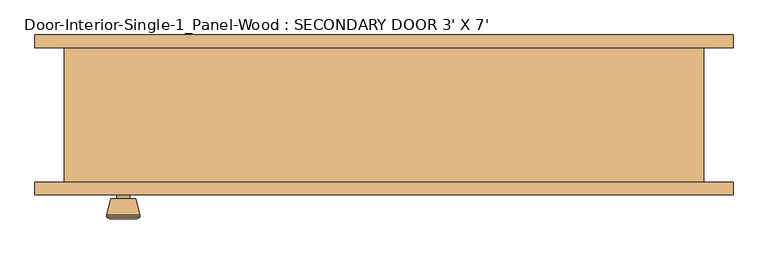
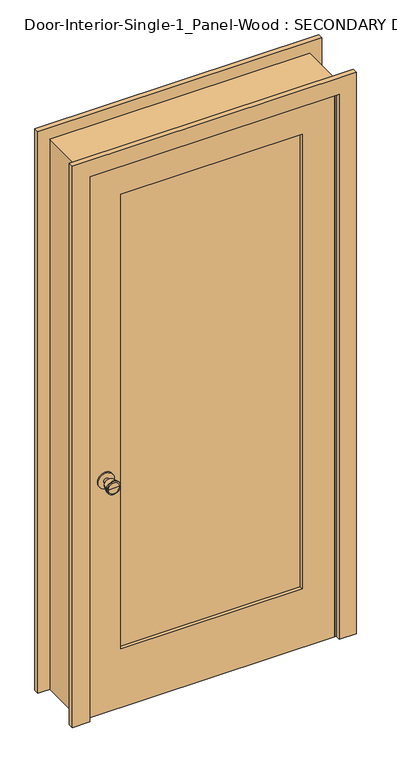
"""IFC4 building model written with IfcOpenShell, lengths in millimetres: door geometry, Door-Interior-Single-1_Panel-Wood : SECONDARY DOOR 3' X 7'."""

from ifc_helpers import new_model, si_unit, point, frame, frame_2d, origin, place, context, project, spatial, polyline, circle_curve, trimmed, segment, composite_curve, outline, extrude, faceted_brep, source, transform, mapped, element, save
from ifc_brep_helpers import plane_surface, cylinder_surface, revolved_surface, advanced_brep


def door_interior_single_1_panel_wood_secondary_door_3_x_7_1a936fe1(model_context):
    return source(origin(), model_context, "Body", "SolidModel", [
        advanced_brep(
        [(-393.7, -57.5, 914.4), (-403.7, -57.5, 914.4), (-383.7, -57.5, 914.4), (-373.2241324, -8.5, 914.4), (-414.1758676, -8.5, 914.4), (-393.7, -8.5, 914.4), (-368.7, -10.3278681, 914.4), (-418.7, -10.3278681, 914.4), (-368.7, -13.7915463, 914.4), (-418.7, -13.7915463, 914.4), (-375.063764, -38.5, 914.4), (-412.336236, -38.5, 914.4), (-383.7, -38.5, 914.4), (-403.7, -38.5, 914.4)],
        [
            (0, 1),
            (1, 2, circle_curve(frame((-393.7, -57.5, 914.4), z_axis=(0.0, -1.0, 0.0), x_axis=(-1.0, 0.0, 0.0)), 10.0)),
            (2, 0),
            (2, 1, circle_curve(frame((-393.7, -57.5, 914.4), z_axis=(0.0, -1.0, 0.0), x_axis=(-1.0, 0.0, 0.0)), 10.0)),
            (3, 4, circle_curve(frame((-393.7, -8.5, 914.4), z_axis=(0.0, 1.0, 0.0), x_axis=(-1.0, 0.0, 0.0)), 20.4758676)),
            (4, 5),
            (5, 3),
            (4, 3, circle_curve(frame((-393.7, -8.5, 914.4), z_axis=(0.0, 1.0, 0.0), x_axis=(-1.0, 0.0, 0.0)), 20.4758676)),
            (6, 7, circle_curve(frame((-393.7, -10.3278681, 914.4), z_axis=(0.0, 1.0, 0.0), x_axis=(-1.0, 0.0, 0.0)), 25.0)),
            (7, 4),
            (3, 6),
            (7, 6, circle_curve(frame((-393.7, -10.3278681, 914.4), z_axis=(0.0, 1.0, 0.0), x_axis=(-1.0, 0.0, 0.0)), 25.0)),
            (8, 9, circle_curve(frame((-393.7, -13.7915463, 914.4), z_axis=(0.0, 1.0, 0.0), x_axis=(-1.0, 0.0, 0.0)), 25.0)),
            (9, 7),
            (6, 8),
            (9, 8, circle_curve(frame((-393.7, -13.7915463, 914.4), z_axis=(0.0, 1.0, 0.0), x_axis=(-1.0, 0.0, 0.0)), 25.0)),
            (10, 11, circle_curve(frame((-393.7, -38.5, 914.4), z_axis=(0.0, 1.0, 0.0), x_axis=(-1.0, 0.0, 0.0)), 18.636236)),
            (11, 9),
            (8, 10),
            (11, 10, circle_curve(frame((-393.7, -38.5, 914.4), z_axis=(0.0, 1.0, 0.0), x_axis=(-1.0, 0.0, 0.0)), 18.636236)),
            (12, 13, circle_curve(frame((-393.7, -38.5, 914.4), z_axis=(0.0, 1.0, 0.0), x_axis=(-1.0, 0.0, 0.0)), 10.0)),
            (13, 11),
            (10, 12),
            (13, 12, circle_curve(frame((-393.7, -38.5, 914.4), z_axis=(0.0, 1.0, 0.0), x_axis=(-1.0, 0.0, 0.0)), 10.0)),
            (1, 13),
            (12, 2),
        ],
        [
            plane_surface(frame((-393.7, -57.5, 914.4), z_axis=(0.0, -1.0, 0.0), x_axis=(-1.0, 0.0, 0.0))),
            plane_surface(frame((-393.7, -8.5, 914.4), z_axis=(0.0, 1.0, 0.0), x_axis=(-1.0, 0.0, 0.0))),
            revolved_surface(polyline([(-414.1758676, -8.5, 914.4), (-418.7, -10.3278681, 914.4)]), (-393.7, -57.5, 914.4), (0.0, -1.0, 0.0)),
            cylinder_surface(frame((-393.7, -57.5, 914.4), z_axis=(0.0, -1.0, 0.0), x_axis=(-1.0, 0.0, 0.0)), 25.0),
            revolved_surface(polyline([(-418.7, -13.7915463, 914.4), (-412.336236, -38.5, 914.4)]), (-393.7, -57.5, 914.4), (0.0, -1.0, 0.0)),
            plane_surface(frame((-393.7, -38.5, 914.4), z_axis=(0.0, -1.0, 0.0), x_axis=(-1.0, 0.0, 0.0))),
            cylinder_surface(frame((-393.7, -57.5, 914.4), z_axis=(0.0, -1.0, 0.0), x_axis=(-1.0, 0.0, 0.0)), 10.0),
        ],
        [
            (0, [[1, 2, 3]]),
            (0, [[-3, 4, -1]]),
            (1, [[5, 6, 7]]),
            (1, [[8, -7, -6]]),
            (2, [[9, 10, -5, 11]]),
            (2, [[12, -11, -8, -10]]),
            (3, [[13, 14, -9, 15]]),
            (3, [[16, -15, -12, -14]]),
            (4, [[17, 18, -13, 19]]),
            (4, [[20, -19, -16, -18]]),
            (5, [[21, 22, -17, 23]]),
            (5, [[24, -23, -20, -22]]),
            (6, [[-2, 25, -21, 26]]),
            (6, [[-4, -26, -24, -25]]),
        ],
    ),
        extrude(outline(composite_curve([segment(trimmed(circle_curve(frame_2d((914.4, -393.7)), 30.0), [point((914.4, -423.7))], [point((914.4, -363.7))], False, "CARTESIAN"), True, "CONTINUOUS"), segment(trimmed(circle_curve(frame_2d((914.4, -393.7)), 30.0), [point((914.4, -363.7))], [point((914.4, -423.7))], False, "CARTESIAN"), True, "CONTINUOUS")], self_intersect=False)), frame((0.0, -63.5, 0.0), z_axis=(0.0, 1.0, 0.0), x_axis=(0.0, 0.0, 1.0)), (0.0, 0.0, 1.0), 6.0),
        advanced_brep(
        [(-393.7, -104.425, 914.4), (-383.7, -104.425, 914.4), (-403.7, -104.425, 914.4), (-373.2241324, -153.425, 914.4), (-393.7, -153.425, 914.4), (-414.1758676, -153.425, 914.4), (-368.7, -151.5971319, 914.4), (-418.7, -151.5971319, 914.4), (-368.7, -148.1334537, 914.4), (-418.7, -148.1334537, 914.4), (-375.063764, -123.425, 914.4), (-412.336236, -123.425, 914.4), (-383.7, -123.425, 914.4), (-403.7, -123.425, 914.4)],
        [
            (0, 1),
            (1, 2, circle_curve(frame((-393.7, -104.425, 914.4), z_axis=(0.0, 1.0, 0.0), x_axis=(-1.0, 0.0, 0.0)), 10.0)),
            (2, 0),
            (2, 1, circle_curve(frame((-393.7, -104.425, 914.4), z_axis=(0.0, 1.0, 0.0), x_axis=(-1.0, 0.0, 0.0)), 10.0)),
            (3, 4),
            (4, 5),
            (5, 3, circle_curve(frame((-393.7, -153.425, 914.4), z_axis=(0.0, -1.0, 0.0), x_axis=(-1.0, 0.0, 0.0)), 20.4758676)),
            (3, 5, circle_curve(frame((-393.7, -153.425, 914.4), z_axis=(0.0, -1.0, 0.0), x_axis=(-1.0, 0.0, 0.0)), 20.4758676)),
            (6, 3),
            (5, 7),
            (7, 6, circle_curve(frame((-393.7, -151.5971319, 914.4), z_axis=(0.0, -1.0, 0.0), x_axis=(-1.0, 0.0, 0.0)), 25.0)),
            (6, 7, circle_curve(frame((-393.7, -151.5971319, 914.4), z_axis=(0.0, -1.0, 0.0), x_axis=(-1.0, 0.0, 0.0)), 25.0)),
            (8, 6),
            (7, 9),
            (9, 8, circle_curve(frame((-393.7, -148.1334537, 914.4), z_axis=(0.0, -1.0, 0.0), x_axis=(-1.0, 0.0, 0.0)), 25.0)),
            (8, 9, circle_curve(frame((-393.7, -148.1334537, 914.4), z_axis=(0.0, -1.0, 0.0), x_axis=(-1.0, 0.0, 0.0)), 25.0)),
            (10, 8),
            (9, 11),
            (11, 10, circle_curve(frame((-393.7, -123.425, 914.4), z_axis=(0.0, -1.0, 0.0), x_axis=(-1.0, 0.0, 0.0)), 18.636236)),
            (10, 11, circle_curve(frame((-393.7, -123.425, 914.4), z_axis=(0.0, -1.0, 0.0), x_axis=(-1.0, 0.0, 0.0)), 18.636236)),
            (12, 10),
            (11, 13),
            (13, 12, circle_curve(frame((-393.7, -123.425, 914.4), z_axis=(0.0, -1.0, 0.0), x_axis=(-1.0, 0.0, 0.0)), 10.0)),
            (12, 13, circle_curve(frame((-393.7, -123.425, 914.4), z_axis=(0.0, -1.0, 0.0), x_axis=(-1.0, 0.0, 0.0)), 10.0)),
            (1, 12),
            (13, 2),
        ],
        [
            plane_surface(frame((-393.7, -104.425, 914.4), z_axis=(0.0, 1.0, 0.0), x_axis=(-1.0, 0.0, 0.0))),
            plane_surface(frame((-393.7, -153.425, 914.4), z_axis=(0.0, -1.0, 0.0), x_axis=(-1.0, 0.0, 0.0))),
            revolved_surface(polyline([(-414.1758676, -153.425, 914.4), (-418.7, -151.5971319, 914.4)]), (-393.7, -104.425, 914.4), (0.0, 1.0, 0.0)),
            cylinder_surface(frame((-393.7, -104.425, 914.4), z_axis=(0.0, 1.0, 0.0), x_axis=(-1.0, 0.0, 0.0)), 25.0),
            revolved_surface(polyline([(-418.7, -148.1334537, 914.4), (-412.336236, -123.425, 914.4)]), (-393.7, -104.425, 914.4), (0.0, 1.0, 0.0)),
            plane_surface(frame((-393.7, -123.425, 914.4), z_axis=(0.0, 1.0, 0.0), x_axis=(-1.0, 0.0, 0.0))),
            cylinder_surface(frame((-393.7, -104.425, 914.4), z_axis=(0.0, 1.0, 0.0), x_axis=(-1.0, 0.0, 0.0)), 10.0),
        ],
        [
            (0, [[1, 2, 3]]),
            (0, [[-3, 4, -1]]),
            (1, [[5, 6, 7]]),
            (1, [[-6, -5, 8]]),
            (2, [[9, -7, 10, 11]]),
            (2, [[-10, -8, -9, 12]]),
            (3, [[13, -11, 14, 15]]),
            (3, [[-14, -12, -13, 16]]),
            (4, [[17, -15, 18, 19]]),
            (4, [[-18, -16, -17, 20]]),
            (5, [[21, -19, 22, 23]]),
            (5, [[-22, -20, -21, 24]]),
            (6, [[25, -23, 26, -2]]),
            (6, [[-26, -24, -25, -4]]),
        ],
    ),
        extrude(outline(composite_curve([segment(trimmed(circle_curve(frame_2d((914.4, -393.7)), 30.0), [point((914.4, -423.7))], [point((914.4, -363.7))], False, "CARTESIAN"), True, "CONTINUOUS"), segment(trimmed(circle_curve(frame_2d((914.4, -393.7)), 30.0), [point((914.4, -363.7))], [point((914.4, -423.7))], False, "CARTESIAN"), True, "CONTINUOUS")], self_intersect=False)), frame((0.0, -104.425, 0.0), z_axis=(0.0, 1.0, 0.0), x_axis=(0.0, 0.0, 1.0)), (0.0, 0.0, 1.0), 6.0),
        faceted_brep([(482.6, -98.425, 0.0), (457.2, -98.425, 0.0), (457.2, -63.5, 0.0), (444.5, -63.5, 0.0), (444.5, -28.575, 0.0), (457.2, -28.575, 0.0), (457.2, 104.775, 0.0), (482.6, 104.775, 0.0), (482.6, 104.775, 2159.0), (482.6, -98.425, 2159.0), (457.2, 104.775, 2133.6), (-457.2, 104.775, 2133.6), (-457.2, 104.775, 0.0), (-482.6, 104.775, 0.0), (-482.6, 104.775, 2159.0), (457.2, -28.575, 2133.6), (444.5, -28.575, 2120.9), (-444.5, -28.575, 2120.9), (-444.5, -28.575, 0.0), (-457.2, -28.575, 0.0), (-457.2, -28.575, 2133.6), (444.5, -63.5, 2120.9), (457.2, -63.5, 2133.6), (-457.2, -63.5, 2133.6), (-457.2, -63.5, 0.0), (-444.5, -63.5, 0.0), (-444.5, -63.5, 2120.9), (457.2, -98.425, 2133.6), (-482.6, -98.425, 2159.0), (-482.6, -98.425, 0.0), (-457.2, -98.425, 0.0), (-457.2, -98.425, 2133.6)], [[[0, 1, 2, 3, 4, 5, 6, 7]], [[7, 8, 9, 0]], [[6, 10, 11, 12, 13, 14, 8, 7]], [[5, 15, 10, 6]], [[4, 16, 17, 18, 19, 20, 15, 5]], [[3, 21, 16, 4]], [[2, 22, 23, 24, 25, 26, 21, 3]], [[1, 27, 22, 2]], [[0, 9, 28, 29, 30, 31, 27, 1]], [[8, 14, 28, 9]], [[15, 20, 11, 10]], [[21, 26, 17, 16]], [[27, 31, 23, 22]], [[29, 13, 12, 19, 18, 25, 24, 30]], [[14, 13, 29, 28]], [[20, 19, 12, 11]], [[26, 25, 18, 17]], [[31, 30, 24, 23]]]),
        extrude(outline(polyline([(2133.6, -457.2), (0.0, -457.2), (0.0, 457.2), (2133.6, 457.2), (2133.6, -457.2)]), holes=[polyline([(2014.5375, -336.55), (2014.5375, 336.55), (231.775, 336.55), (231.775, -336.55), (2014.5375, -336.55)])]), frame((0.0, -98.425, 0.0), z_axis=(0.0, 1.0, 0.0), x_axis=(0.0, 0.0, 1.0)), (0.0, 0.0, 1.0), 34.925),
        extrude(outline(polyline([(336.55, -75.1416667), (336.55, -86.7833333), (-336.55, -86.7833333), (-336.55, -75.1416667), (336.55, -75.1416667)])), frame((0.0, 0.0, 231.775), z_axis=(0.0, 0.0, 1.0), x_axis=(1.0, 0.0, 0.0)), (0.0, 0.0, 1.0), 1782.7625),
        extrude(outline(polyline([(0.0, 527.05), (2203.45, 527.05), (2203.45, -527.05), (0.0, -527.05), (0.0, -463.55), (2139.95, -463.55), (2139.95, 463.55), (0.0, 463.55), (0.0, 527.05)])), frame((0.0, -117.475, 0.0), z_axis=(0.0, 1.0, 0.0), x_axis=(0.0, 0.0, 1.0)), (0.0, 0.0, 1.0), 19.05),
        extrude(outline(polyline([(0.0, 527.05), (2203.45, 527.05), (2203.45, -527.05), (0.0, -527.05), (0.0, -463.55), (2139.95, -463.55), (2139.95, 463.55), (0.0, 463.55), (0.0, 527.05)])), frame((0.0, 104.775, 0.0), z_axis=(0.0, 1.0, 0.0), x_axis=(0.0, 0.0, 1.0)), (0.0, 0.0, 1.0), 19.05),
    ])


if __name__ == "__main__":
    model = new_model("IFC4")
    model_context = context("Model", 3, world=origin())
    ifc_project = project(units=[si_unit("LENGTHUNIT", "METRE", prefix="MILLI")], contexts=[model_context])
    site = spatial("IfcSite", under=ifc_project)
    building = spatial("IfcBuilding", under=site)
    placement = place(None, origin())
    door_interior_single_1_panel_wood_secondary_door_3_x_7_shape = door_interior_single_1_panel_wood_secondary_door_3_x_7_1a936fe1(model_context)
    element("IfcDoor", 1, ObjectType="Door-Interior-Single-1_Panel-Wood : SECONDARY DOOR 3' X 7'", at=placement, inside=building, context=model_context, shape_type="MappedRepresentation", body=[
        mapped(door_interior_single_1_panel_wood_secondary_door_3_x_7_shape, transform((0.0, 0.0, 0.0), x_axis=(1.0, 0.0, 0.0), y_axis=(0.0, 1.0, 0.0), z_axis=(0.0, 0.0, 1.0))),
    ])
    save(model, "model.ifc")

# Revit data of these elements
# Type "Door-Interior-Single-1_Panel-Wood : SECONDARY DOOR 3' X 7'"
#   Type Mark = "11"
#   Assembly Code = "C1020300"
#   Analytic Construction = "Wooden"
#   Top Rail = 0' - 4 11/16"
#   Thickness = 0' - 1 3/8"
#   Thermal Resistance (R) = 2.5876 (h·ft²·°F)/BTU
#   Swing Angle [instance default] = 90.00°
#   Stiles = 0' - 4 3/4"
#   Rough Width = 3' - 2"
#   Rough Height = 7' - 1"
#   Height = 7' - 0"
#   Width = 3' - 0"
#   Heat Transfer Coefficient (U) = 0.3865 BTU/(h·ft²·°F)
#   Bottom Rail = 0' - 9 1/8"
#   Trim Material = Cherry
#   Panel Material = Cherry
#   Frame Material = Cherry
#   Door Handle Material = Aluminum
#   Visual Light Transmittance = 0
#   Solar Heat Gain Coefficient = 0
#   Wall Closure = (empty or 0)
#   Function = (empty or 0)
# Element 1 (IfcDoor, "Door-Interior-Single-1_Panel-Wood : SECONDARY DOOR 3' X 7'")
#   Materials on its faces: "Cherry", "Aluminum"
# Materials
#   "Cherry": class "Wood", colour RGB 226 177 128, transparency 0, Description = "Prunus Serotina", Cost = 0
#   "Aluminum": class "Metal", colour RGB 247 247 247, transparency 0, Description = "Aluminum 6061", Cost = 0
